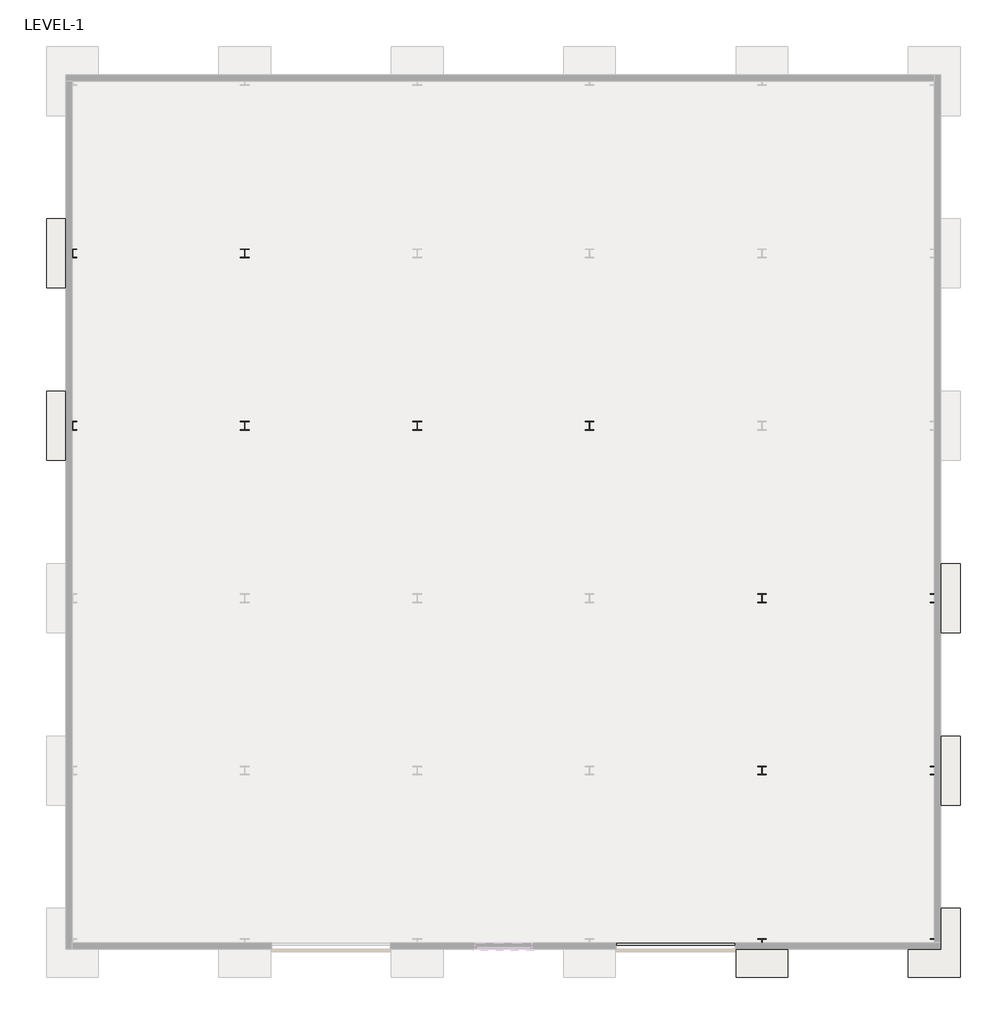
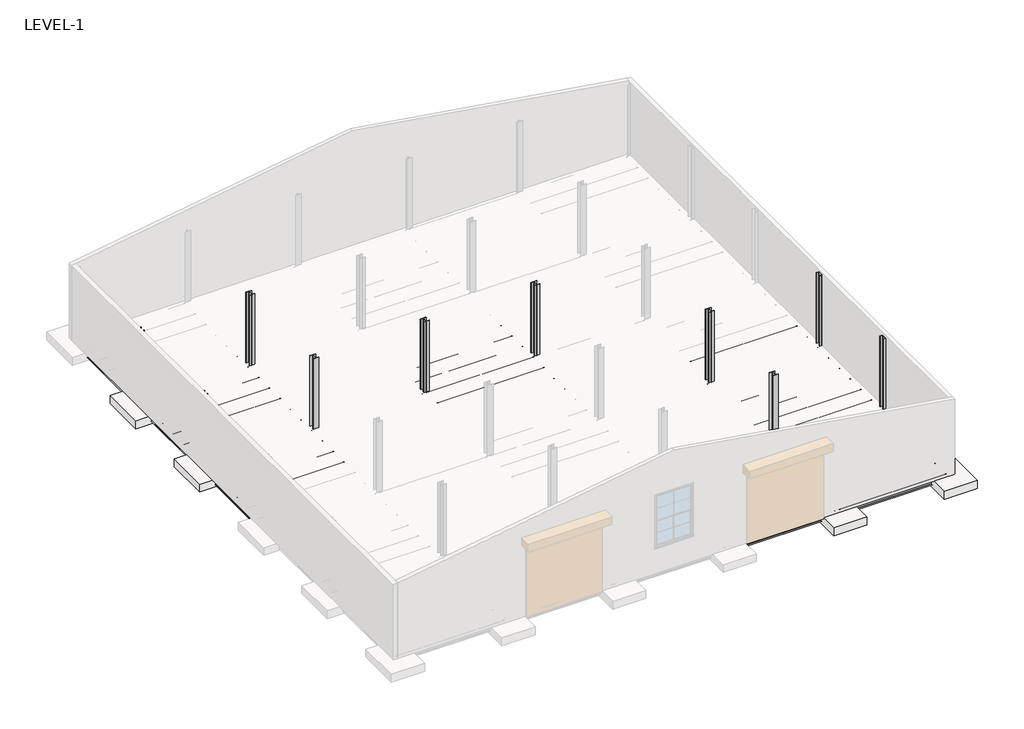
# One storey, part 2 of 3: 70 beams, 12 columns, 12 slabs.
"""IFC4 building model written with IfcOpenShell, lengths in millimetres."""

from ifc_helpers import new_model, si_unit, origin, place, context, project, spatial, transform, mapped, element, save
from components import ub_universal_beams_ub305x165x40_15f88fa9, ub_universal_beams_ub305x165x40_f918ae41, ub_universal_beams_ub305x165x40_f15b2736, ub_universal_beams_ub305x165x40_694d595e, ub_universal_beams_ub305x165x40_db4e7ae9, uc_universal_columns_column_uc305x305x97_11a20181, slab_7b69f09a

model = new_model("IFC4")

# Units and contexts
model_context = context("Model", 3, world=origin())
ifc_project = project(units=[si_unit("LENGTHUNIT", "METRE", prefix="MILLI")], contexts=[model_context])

# Site, building, storey
site = spatial("IfcSite", under=ifc_project)
building = spatial("IfcBuilding", under=site)
storey = spatial("IfcBuildingStorey", under=building, Name="LEVEL-1", Elevation=0.0)

# Beams
placement = place(None, origin())
ub_universal_beams_ub305x165x40_shape = ub_universal_beams_ub305x165x40_15f88fa9(model_context)
element("IfcBeam", 1, ObjectType="UB-Universal Beams : UB305x165x40", at=placement, inside=storey, context=model_context, shape_type="MappedRepresentation", body=[
    mapped(ub_universal_beams_ub305x165x40_shape, transform((-15492.3332854, 11071.5234105, -151.7), x_axis=(1.0, 0.0, 0.0), y_axis=(0.0, 1.0, 0.0), z_axis=(0.0, 0.0, 1.0))),
])
element("IfcBeam", 2, ObjectType="UB-Universal Beams : UB305x165x40", at=placement, inside=storey, context=model_context, shape_type="MappedRepresentation", body=[
    mapped(ub_universal_beams_ub305x165x40_shape, transform((-15492.3332854, 9039.5234105, -151.7), x_axis=(1.0, 0.0, 0.0), y_axis=(0.0, 1.0, 0.0), z_axis=(0.0, 0.0, 1.0))),
])
element("IfcBeam", 3, ObjectType="UB-Universal Beams : UB305x165x40", at=placement, inside=storey, context=model_context, shape_type="MappedRepresentation", body=[
    mapped(ub_universal_beams_ub305x165x40_shape, transform((-15492.3332854, 8023.5234105, -151.7), x_axis=(1.0, 0.0, 0.0), y_axis=(0.0, 1.0, 0.0), z_axis=(0.0, 0.0, 1.0))),
])
element("IfcBeam", 4, ObjectType="UB-Universal Beams : UB305x165x40", at=placement, inside=storey, context=model_context, shape_type="MappedRepresentation", body=[
    mapped(ub_universal_beams_ub305x165x40_shape, transform((-15492.3332854, 7007.5234105, -151.7), x_axis=(1.0, 0.0, 0.0), y_axis=(0.0, 1.0, 0.0), z_axis=(0.0, 0.0, 1.0))),
])
element("IfcBeam", 5, ObjectType="UB-Universal Beams : UB305x165x40", at=placement, inside=storey, context=model_context, shape_type="MappedRepresentation", body=[
    mapped(ub_universal_beams_ub305x165x40_shape, transform((-15492.3332854, 5991.5234105, -151.7), x_axis=(1.0, 0.0, 0.0), y_axis=(0.0, 1.0, 0.0), z_axis=(0.0, 0.0, 1.0))),
])
element("IfcBeam", 6, ObjectType="UB-Universal Beams : UB305x165x40", at=placement, inside=storey, context=model_context, shape_type="MappedRepresentation", body=[
    mapped(ub_universal_beams_ub305x165x40_shape, transform((-15492.3332854, 4975.5234105, -151.7), x_axis=(1.0, 0.0, 0.0), y_axis=(0.0, 1.0, 0.0), z_axis=(0.0, 0.0, 1.0))),
])
element("IfcBeam", 7, ObjectType="UB-Universal Beams : UB305x165x40", at=placement, inside=storey, context=model_context, shape_type="MappedRepresentation", body=[
    mapped(ub_universal_beams_ub305x165x40_shape, transform((-15492.3332854, 2943.5234105, -151.7), x_axis=(1.0, 0.0, 0.0), y_axis=(0.0, 1.0, 0.0), z_axis=(0.0, 0.0, 1.0))),
])
element("IfcBeam", 8, ObjectType="UB-Universal Beams : UB305x165x40", at=placement, inside=storey, context=model_context, shape_type="MappedRepresentation", body=[
    mapped(ub_universal_beams_ub305x165x40_shape, transform((-15492.3332854, 1927.5234105, -151.7), x_axis=(1.0, 0.0, 0.0), y_axis=(0.0, 1.0, 0.0), z_axis=(0.0, 0.0, 1.0))),
])
element("IfcBeam", 9, ObjectType="UB-Universal Beams : UB305x165x40", at=placement, inside=storey, context=model_context, shape_type="MappedRepresentation", body=[
    mapped(ub_universal_beams_ub305x165x40_shape, transform((-15492.3332854, 911.5234105, -151.7), x_axis=(1.0, 0.0, 0.0), y_axis=(0.0, 1.0, 0.0), z_axis=(0.0, 0.0, 1.0))),
])
element("IfcBeam", 10, ObjectType="UB-Universal Beams : UB305x165x40", at=placement, inside=storey, context=model_context, shape_type="MappedRepresentation", body=[
    mapped(ub_universal_beams_ub305x165x40_shape, transform((-3300.3332854, 7007.5234105, -151.7), x_axis=(1.0, 0.0, 0.0), y_axis=(0.0, 1.0, 0.0), z_axis=(0.0, 0.0, 1.0))),
])
element("IfcBeam", 11, ObjectType="UB-Universal Beams : UB305x165x40", at=placement, inside=storey, context=model_context, shape_type="MappedRepresentation", body=[
    mapped(ub_universal_beams_ub305x165x40_shape, transform((-3300.3332854, 5991.5234105, -151.7), x_axis=(1.0, 0.0, 0.0), y_axis=(0.0, 1.0, 0.0), z_axis=(0.0, 0.0, 1.0))),
])
element("IfcBeam", 12, ObjectType="UB-Universal Beams : UB305x165x40", at=placement, inside=storey, context=model_context, shape_type="MappedRepresentation", body=[
    mapped(ub_universal_beams_ub305x165x40_shape, transform((-3300.3332854, 4975.5234105, -151.7), x_axis=(1.0, 0.0, 0.0), y_axis=(0.0, 1.0, 0.0), z_axis=(0.0, 0.0, 1.0))),
])
element("IfcBeam", 13, ObjectType="UB-Universal Beams : UB305x165x40", at=placement, inside=storey, context=model_context, shape_type="MappedRepresentation", body=[
    mapped(ub_universal_beams_ub305x165x40_shape, transform((-3300.3332854, 2943.5234105, -151.7), x_axis=(1.0, 0.0, 0.0), y_axis=(0.0, 1.0, 0.0), z_axis=(0.0, 0.0, 1.0))),
])
element("IfcBeam", 14, ObjectType="UB-Universal Beams : UB305x165x40", at=placement, inside=storey, context=model_context, shape_type="MappedRepresentation", body=[
    mapped(ub_universal_beams_ub305x165x40_shape, transform((-3300.3332854, 1927.5234105, -151.7), x_axis=(1.0, 0.0, 0.0), y_axis=(0.0, 1.0, 0.0), z_axis=(0.0, 0.0, 1.0))),
])
element("IfcBeam", 15, ObjectType="UB-Universal Beams : UB305x165x40", at=placement, inside=storey, context=model_context, shape_type="MappedRepresentation", body=[
    mapped(ub_universal_beams_ub305x165x40_shape, transform((-3300.3332854, 911.5234105, -151.7), x_axis=(1.0, 0.0, 0.0), y_axis=(0.0, 1.0, 0.0), z_axis=(0.0, 0.0, 1.0))),
])
element("IfcBeam", 16, ObjectType="UB-Universal Beams : UB305x165x40", at=placement, inside=storey, context=model_context, shape_type="MappedRepresentation", body=[
    mapped(ub_universal_beams_ub305x165x40_shape, transform((8891.6667146, -104.4765895, -151.7), x_axis=(1.0, 0.0, 0.0), y_axis=(0.0, 1.0, 0.0), z_axis=(0.0, 0.0, 1.0))),
])
element("IfcBeam", 17, ObjectType="UB-Universal Beams : UB305x165x40", at=placement, inside=storey, context=model_context, shape_type="MappedRepresentation", body=[
    mapped(ub_universal_beams_ub305x165x40_shape, transform((8891.6667146, -1120.4765895, -151.7), x_axis=(1.0, 0.0, 0.0), y_axis=(0.0, 1.0, 0.0), z_axis=(0.0, 0.0, 1.0))),
])
element("IfcBeam", 18, ObjectType="UB-Universal Beams : UB305x165x40", at=placement, inside=storey, context=model_context, shape_type="MappedRepresentation", body=[
    mapped(ub_universal_beams_ub305x165x40_shape, transform((8891.6667146, -3152.4765895, -151.7), x_axis=(1.0, 0.0, 0.0), y_axis=(0.0, 1.0, 0.0), z_axis=(0.0, 0.0, 1.0))),
])
element("IfcBeam", 19, ObjectType="UB-Universal Beams : UB305x165x40", at=placement, inside=storey, context=model_context, shape_type="MappedRepresentation", body=[
    mapped(ub_universal_beams_ub305x165x40_shape, transform((8891.6667146, -4168.4765895, -151.7), x_axis=(1.0, 0.0, 0.0), y_axis=(0.0, 1.0, 0.0), z_axis=(0.0, 0.0, 1.0))),
])
element("IfcBeam", 20, ObjectType="UB-Universal Beams : UB305x165x40", at=placement, inside=storey, context=model_context, shape_type="MappedRepresentation", body=[
    mapped(ub_universal_beams_ub305x165x40_shape, transform((8891.6667146, -5184.4765895, -151.7), x_axis=(1.0, 0.0, 0.0), y_axis=(0.0, 1.0, 0.0), z_axis=(0.0, 0.0, 1.0))),
])
element("IfcBeam", 21, ObjectType="UB-Universal Beams : UB305x165x40", at=placement, inside=storey, context=model_context, shape_type="MappedRepresentation", body=[
    mapped(ub_universal_beams_ub305x165x40_shape, transform((8891.6667146, -6200.4765895, -151.7), x_axis=(1.0, 0.0, 0.0), y_axis=(0.0, 1.0, 0.0), z_axis=(0.0, 0.0, 1.0))),
])
element("IfcBeam", 22, ObjectType="UB-Universal Beams : UB305x165x40", at=placement, inside=storey, context=model_context, shape_type="MappedRepresentation", body=[
    mapped(ub_universal_beams_ub305x165x40_shape, transform((8891.6667146, -7216.4765895, -151.7), x_axis=(1.0, 0.0, 0.0), y_axis=(0.0, 1.0, 0.0), z_axis=(0.0, 0.0, 1.0))),
])
element("IfcBeam", 23, ObjectType="UB-Universal Beams : UB305x165x40", at=placement, inside=storey, context=model_context, shape_type="MappedRepresentation", body=[
    mapped(ub_universal_beams_ub305x165x40_shape, transform((8891.6667146, -9248.4765895, -151.7), x_axis=(1.0, 0.0, 0.0), y_axis=(0.0, 1.0, 0.0), z_axis=(0.0, 0.0, 1.0))),
])
element("IfcBeam", 24, ObjectType="UB-Universal Beams : UB305x165x40", at=placement, inside=storey, context=model_context, shape_type="MappedRepresentation", body=[
    mapped(ub_universal_beams_ub305x165x40_shape, transform((8891.6667146, -10264.4765895, -151.7), x_axis=(1.0, 0.0, 0.0), y_axis=(0.0, 1.0, 0.0), z_axis=(0.0, 0.0, 1.0))),
])
element("IfcBeam", 25, ObjectType="UB-Universal Beams : UB305x165x40", at=placement, inside=storey, context=model_context, shape_type="MappedRepresentation", body=[
    mapped(ub_universal_beams_ub305x165x40_shape, transform((8891.6667146, -11280.4765895, -151.7), x_axis=(1.0, 0.0, 0.0), y_axis=(0.0, 1.0, 0.0), z_axis=(0.0, 0.0, 1.0))),
])
element("IfcBeam", 26, ObjectType="UB-Universal Beams : UB305x165x40", at=placement, inside=storey, context=model_context, shape_type="MappedRepresentation", body=[
    mapped(ub_universal_beams_ub305x165x40_shape, transform((8891.6667146, -12296.4765895, -151.7), x_axis=(1.0, 0.0, 0.0), y_axis=(0.0, 1.0, 0.0), z_axis=(0.0, 0.0, 1.0))),
])
element("IfcBeam", 27, ObjectType="UB-Universal Beams : UB305x165x40", at=placement, inside=storey, context=model_context, shape_type="MappedRepresentation", body=[
    mapped(ub_universal_beams_ub305x165x40_shape, transform((8891.6667146, -13312.4765895, -151.7), x_axis=(1.0, 0.0, 0.0), y_axis=(0.0, 1.0, 0.0), z_axis=(0.0, 0.0, 1.0))),
])
element("IfcBeam", 28, ObjectType="UB-Universal Beams : UB305x165x40", at=placement, inside=storey, context=model_context, shape_type="MappedRepresentation", body=[
    mapped(ub_universal_beams_ub305x165x40_shape, transform((-7364.3332854, 7007.5234105, -151.7), x_axis=(0.0, -1.0, 0.0), y_axis=(1.0, 0.0, 0.0), z_axis=(0.0, 0.0, 1.0))),
])
element("IfcBeam", 29, ObjectType="UB-Universal Beams : UB305x165x40", at=placement, inside=storey, context=model_context, shape_type="MappedRepresentation", body=[
    mapped(ub_universal_beams_ub305x165x40_shape, transform((-8380.3332854, 7007.5234105, -151.7), x_axis=(0.0, -1.0, 0.0), y_axis=(1.0, 0.0, 0.0), z_axis=(0.0, 0.0, 1.0))),
])
element("IfcBeam", 30, ObjectType="UB-Universal Beams : UB305x165x40", at=placement, inside=storey, context=model_context, shape_type="MappedRepresentation", body=[
    mapped(ub_universal_beams_ub305x165x40_shape, transform((-9396.3332854, 7007.5234105, -151.7), x_axis=(0.0, -1.0, 0.0), y_axis=(1.0, 0.0, 0.0), z_axis=(0.0, 0.0, 1.0))),
])
element("IfcBeam", 31, ObjectType="UB-Universal Beams : UB305x165x40", at=placement, inside=storey, context=model_context, shape_type="MappedRepresentation", body=[
    mapped(ub_universal_beams_ub305x165x40_shape, transform((-10412.3332854, 7007.5234105, -151.7), x_axis=(0.0, -1.0, 0.0), y_axis=(1.0, 0.0, 0.0), z_axis=(0.0, 0.0, 1.0))),
])
element("IfcBeam", 32, ObjectType="UB-Universal Beams : UB305x165x40", at=placement, inside=storey, context=model_context, shape_type="MappedRepresentation", body=[
    mapped(ub_universal_beams_ub305x165x40_shape, transform((-11428.3332854, 7007.5234105, -151.7), x_axis=(0.0, -1.0, 0.0), y_axis=(1.0, 0.0, 0.0), z_axis=(0.0, 0.0, 1.0))),
])
element("IfcBeam", 33, ObjectType="UB-Universal Beams : UB305x165x40", at=placement, inside=storey, context=model_context, shape_type="MappedRepresentation", body=[
    mapped(ub_universal_beams_ub305x165x40_shape, transform((-7364.3332854, 911.5234105, -151.7), x_axis=(0.0, -1.0, 0.0), y_axis=(1.0, 0.0, 0.0), z_axis=(0.0, 0.0, 1.0))),
])
element("IfcBeam", 34, ObjectType="UB-Universal Beams : UB305x165x40", at=placement, inside=storey, context=model_context, shape_type="MappedRepresentation", body=[
    mapped(ub_universal_beams_ub305x165x40_shape, transform((-8380.3332854, 911.5234105, -151.7), x_axis=(0.0, -1.0, 0.0), y_axis=(1.0, 0.0, 0.0), z_axis=(0.0, 0.0, 1.0))),
])
element("IfcBeam", 35, ObjectType="UB-Universal Beams : UB305x165x40", at=placement, inside=storey, context=model_context, shape_type="MappedRepresentation", body=[
    mapped(ub_universal_beams_ub305x165x40_shape, transform((-9396.3332854, 911.5234105, -151.7), x_axis=(0.0, -1.0, 0.0), y_axis=(1.0, 0.0, 0.0), z_axis=(0.0, 0.0, 1.0))),
])
element("IfcBeam", 36, ObjectType="UB-Universal Beams : UB305x165x40", at=placement, inside=storey, context=model_context, shape_type="MappedRepresentation", body=[
    mapped(ub_universal_beams_ub305x165x40_shape, transform((-10412.3332854, 911.5234105, -151.7), x_axis=(0.0, -1.0, 0.0), y_axis=(1.0, 0.0, 0.0), z_axis=(0.0, 0.0, 1.0))),
])
element("IfcBeam", 37, ObjectType="UB-Universal Beams : UB305x165x40", at=placement, inside=storey, context=model_context, shape_type="MappedRepresentation", body=[
    mapped(ub_universal_beams_ub305x165x40_shape, transform((-11428.3332854, 911.5234105, -151.7), x_axis=(0.0, -1.0, 0.0), y_axis=(1.0, 0.0, 0.0), z_axis=(0.0, 0.0, 1.0))),
])
element("IfcBeam", 38, ObjectType="UB-Universal Beams : UB305x165x40", at=placement, inside=storey, context=model_context, shape_type="MappedRepresentation", body=[
    mapped(ub_universal_beams_ub305x165x40_shape, transform((4827.6667146, -5184.4765895, -151.7), x_axis=(0.0, -1.0, 0.0), y_axis=(1.0, 0.0, 0.0), z_axis=(0.0, 0.0, 1.0))),
])
element("IfcBeam", 39, ObjectType="UB-Universal Beams : UB305x165x40", at=placement, inside=storey, context=model_context, shape_type="MappedRepresentation", body=[
    mapped(ub_universal_beams_ub305x165x40_shape, transform((3811.6667146, -5184.4765895, -151.7), x_axis=(0.0, -1.0, 0.0), y_axis=(1.0, 0.0, 0.0), z_axis=(0.0, 0.0, 1.0))),
])
element("IfcBeam", 40, ObjectType="UB-Universal Beams : UB305x165x40", at=placement, inside=storey, context=model_context, shape_type="MappedRepresentation", body=[
    mapped(ub_universal_beams_ub305x165x40_shape, transform((2795.6667146, -5184.4765895, -151.7), x_axis=(0.0, -1.0, 0.0), y_axis=(1.0, 0.0, 0.0), z_axis=(0.0, 0.0, 1.0))),
])
element("IfcBeam", 41, ObjectType="UB-Universal Beams : UB305x165x40", at=placement, inside=storey, context=model_context, shape_type="MappedRepresentation", body=[
    mapped(ub_universal_beams_ub305x165x40_shape, transform((1779.6667146, -5184.4765895, -151.7), x_axis=(0.0, -1.0, 0.0), y_axis=(1.0, 0.0, 0.0), z_axis=(0.0, 0.0, 1.0))),
])
element("IfcBeam", 42, ObjectType="UB-Universal Beams : UB305x165x40", at=placement, inside=storey, context=model_context, shape_type="MappedRepresentation", body=[
    mapped(ub_universal_beams_ub305x165x40_shape, transform((763.6667146, -5184.4765895, -151.7), x_axis=(0.0, -1.0, 0.0), y_axis=(1.0, 0.0, 0.0), z_axis=(0.0, 0.0, 1.0))),
])
element("IfcBeam", 43, ObjectType="UB-Universal Beams : UB305x165x40", at=placement, inside=storey, context=model_context, shape_type="MappedRepresentation", body=[
    mapped(ub_universal_beams_ub305x165x40_shape, transform((4827.6667146, -11280.4765895, -151.7), x_axis=(0.0, -1.0, 0.0), y_axis=(1.0, 0.0, 0.0), z_axis=(0.0, 0.0, 1.0))),
])
element("IfcBeam", 44, ObjectType="UB-Universal Beams : UB305x165x40", at=placement, inside=storey, context=model_context, shape_type="MappedRepresentation", body=[
    mapped(ub_universal_beams_ub305x165x40_shape, transform((3811.6667146, -11280.4765895, -151.7), x_axis=(0.0, -1.0, 0.0), y_axis=(1.0, 0.0, 0.0), z_axis=(0.0, 0.0, 1.0))),
])
element("IfcBeam", 45, ObjectType="UB-Universal Beams : UB305x165x40", at=placement, inside=storey, context=model_context, shape_type="MappedRepresentation", body=[
    mapped(ub_universal_beams_ub305x165x40_shape, transform((2795.6667146, -11280.4765895, -151.7), x_axis=(0.0, -1.0, 0.0), y_axis=(1.0, 0.0, 0.0), z_axis=(0.0, 0.0, 1.0))),
])
element("IfcBeam", 46, ObjectType="UB-Universal Beams : UB305x165x40", at=placement, inside=storey, context=model_context, shape_type="MappedRepresentation", body=[
    mapped(ub_universal_beams_ub305x165x40_shape, transform((1779.6667146, -11280.4765895, -151.7), x_axis=(0.0, -1.0, 0.0), y_axis=(1.0, 0.0, 0.0), z_axis=(0.0, 0.0, 1.0))),
])
element("IfcBeam", 47, ObjectType="UB-Universal Beams : UB305x165x40", at=placement, inside=storey, context=model_context, shape_type="MappedRepresentation", body=[
    mapped(ub_universal_beams_ub305x165x40_shape, transform((763.6667146, -11280.4765895, -151.7), x_axis=(0.0, -1.0, 0.0), y_axis=(1.0, 0.0, 0.0), z_axis=(0.0, 0.0, 1.0))),
])
element("IfcBeam", 48, ObjectType="UB-Universal Beams : UB305x165x40", at=placement, inside=storey, context=model_context, shape_type="MappedRepresentation", body=[
    mapped(ub_universal_beams_ub305x165x40_shape, transform((2795.6667146, -14328.4765895, -151.7), x_axis=(1.0, 0.0, 0.0), y_axis=(0.0, 1.0, 0.0), z_axis=(0.0, 0.0, 1.0))),
])
element("IfcBeam", 49, ObjectType="UB-Universal Beams : UB305x165x40", at=placement, inside=storey, context=model_context, shape_type="MappedRepresentation", body=[
    mapped(ub_universal_beams_ub305x165x40_shape, transform((8891.6667146, -14328.4765895, -151.7), x_axis=(1.0, 0.0, 0.0), y_axis=(0.0, 1.0, 0.0), z_axis=(0.0, 0.0, 1.0))),
])
element("IfcBeam", 50, ObjectType="UB-Universal Beams : UB305x165x40", at=placement, inside=storey, context=model_context, shape_type="MappedRepresentation", body=[
    mapped(ub_universal_beams_ub305x165x40_shape, transform((2795.6667146, -8232.4765895, -151.7), x_axis=(1.0, 0.0, 0.0), y_axis=(0.0, 1.0, 0.0), z_axis=(0.0, 0.0, 1.0))),
])
element("IfcBeam", 51, ObjectType="UB-Universal Beams : UB305x165x40", at=placement, inside=storey, context=model_context, shape_type="MappedRepresentation", body=[
    mapped(ub_universal_beams_ub305x165x40_shape, transform((8891.6667146, -8232.4765895, -151.7), x_axis=(1.0, 0.0, 0.0), y_axis=(0.0, 1.0, 0.0), z_axis=(0.0, 0.0, 1.0))),
])
element("IfcBeam", 52, ObjectType="UB-Universal Beams : UB305x165x40", at=placement, inside=storey, context=model_context, shape_type="MappedRepresentation", body=[
    mapped(ub_universal_beams_ub305x165x40_shape, transform((2795.6667146, -2136.4765895, -151.7), x_axis=(1.0, 0.0, 0.0), y_axis=(0.0, 1.0, 0.0), z_axis=(0.0, 0.0, 1.0))),
])
element("IfcBeam", 53, ObjectType="UB-Universal Beams : UB305x165x40", at=placement, inside=storey, context=model_context, shape_type="MappedRepresentation", body=[
    mapped(ub_universal_beams_ub305x165x40_shape, transform((8891.6667146, -2136.4765895, -151.7), x_axis=(1.0, 0.0, 0.0), y_axis=(0.0, 1.0, 0.0), z_axis=(0.0, 0.0, 1.0))),
])
element("IfcBeam", 54, ObjectType="UB-Universal Beams : UB305x165x40", at=placement, inside=storey, context=model_context, shape_type="MappedRepresentation", body=[
    mapped(ub_universal_beams_ub305x165x40_shape, transform((-9396.3332854, 3959.5234105, -151.7), x_axis=(1.0, 0.0, 0.0), y_axis=(0.0, 1.0, 0.0), z_axis=(0.0, 0.0, 1.0))),
])
element("IfcBeam", 55, ObjectType="UB-Universal Beams : UB305x165x40", at=placement, inside=storey, context=model_context, shape_type="MappedRepresentation", body=[
    mapped(ub_universal_beams_ub305x165x40_shape, transform((-3300.3332854, 3959.5234105, -151.7), x_axis=(1.0, 0.0, 0.0), y_axis=(0.0, 1.0, 0.0), z_axis=(0.0, 0.0, 1.0))),
])
element("IfcBeam", 56, ObjectType="UB-Universal Beams : UB305x165x40", at=placement, inside=storey, context=model_context, shape_type="MappedRepresentation", body=[
    mapped(ub_universal_beams_ub305x165x40_shape, transform((-18540.3332854, 911.5234105, -151.7), x_axis=(0.0, 1.0, 0.0), y_axis=(-1.0, 0.0, 0.0), z_axis=(0.0, 0.0, 1.0))),
])
element("IfcBeam", 57, ObjectType="UB-Universal Beams : UB305x165x40", at=placement, inside=storey, context=model_context, shape_type="MappedRepresentation", body=[
    mapped(ub_universal_beams_ub305x165x40_shape, transform((-18540.3332854, 7007.5234105, -151.7), x_axis=(0.0, 1.0, 0.0), y_axis=(-1.0, 0.0, 0.0), z_axis=(0.0, 0.0, 1.0))),
])
ub_universal_beams_ub305x165x40_2_shape = ub_universal_beams_ub305x165x40_f918ae41(model_context)
element("IfcBeam", 58, ObjectType="UB-Universal Beams : UB305x165x40", at=placement, inside=storey, context=model_context, shape_type="MappedRepresentation", body=[
    mapped(ub_universal_beams_ub305x165x40_2_shape, transform((11939.6667146, -5184.4765895, -151.7), x_axis=(0.0, 1.0, 0.0), y_axis=(-1.0, 0.0, 0.0), z_axis=(0.0, 0.0, 1.0))),
])
element("IfcBeam", 59, ObjectType="UB-Universal Beams : UB305x165x40", at=placement, inside=storey, context=model_context, shape_type="MappedRepresentation", body=[
    mapped(ub_universal_beams_ub305x165x40_2_shape, transform((5843.6667146, -5184.4765895, -151.7), x_axis=(0.0, 1.0, 0.0), y_axis=(-1.0, 0.0, 0.0), z_axis=(0.0, 0.0, 1.0))),
])
element("IfcBeam", 60, ObjectType="UB-Universal Beams : UB305x165x40", at=placement, inside=storey, context=model_context, shape_type="MappedRepresentation", body=[
    mapped(ub_universal_beams_ub305x165x40_2_shape, transform((-252.3332854, 911.5234105, -151.7), x_axis=(0.0, 1.0, 0.0), y_axis=(-1.0, 0.0, 0.0), z_axis=(0.0, 0.0, 1.0))),
])
element("IfcBeam", 61, ObjectType="UB-Universal Beams : UB305x165x40", at=placement, inside=storey, context=model_context, shape_type="MappedRepresentation", body=[
    mapped(ub_universal_beams_ub305x165x40_2_shape, transform((-252.3332854, 7007.5234105, -151.7), x_axis=(0.0, 1.0, 0.0), y_axis=(-1.0, 0.0, 0.0), z_axis=(0.0, 0.0, 1.0))),
])
element("IfcBeam", 62, ObjectType="UB-Universal Beams : UB305x165x40", at=placement, inside=storey, context=model_context, shape_type="MappedRepresentation", body=[
    mapped(ub_universal_beams_ub305x165x40_2_shape, transform((-6348.3332854, 911.5234105, -151.7), x_axis=(0.0, 1.0, 0.0), y_axis=(-1.0, 0.0, 0.0), z_axis=(0.0, 0.0, 1.0))),
])
element("IfcBeam", 63, ObjectType="UB-Universal Beams : UB305x165x40", at=placement, inside=storey, context=model_context, shape_type="MappedRepresentation", body=[
    mapped(ub_universal_beams_ub305x165x40_2_shape, transform((-6348.3332854, 7007.5234105, -151.7), x_axis=(0.0, 1.0, 0.0), y_axis=(-1.0, 0.0, 0.0), z_axis=(0.0, 0.0, 1.0))),
])
element("IfcBeam", 64, ObjectType="UB-Universal Beams : UB305x165x40", at=placement, inside=storey, context=model_context, shape_type="MappedRepresentation", body=[
    mapped(ub_universal_beams_ub305x165x40_2_shape, transform((-12444.3332854, 911.5234105, -151.7), x_axis=(0.0, 1.0, 0.0), y_axis=(-1.0, 0.0, 0.0), z_axis=(0.0, 0.0, 1.0))),
])
element("IfcBeam", 65, ObjectType="UB-Universal Beams : UB305x165x40", at=placement, inside=storey, context=model_context, shape_type="MappedRepresentation", body=[
    mapped(ub_universal_beams_ub305x165x40_2_shape, transform((-12444.3332854, 7007.5234105, -151.7), x_axis=(0.0, 1.0, 0.0), y_axis=(-1.0, 0.0, 0.0), z_axis=(0.0, 0.0, 1.0))),
])
ub_universal_beams_ub305x165x40_3_shape = ub_universal_beams_ub305x165x40_f15b2736(model_context)
element("IfcBeam", 66, ObjectType="UB-Universal Beams : UB305x165x40", at=placement, inside=storey, context=model_context, shape_type="MappedRepresentation", body=[
    mapped(ub_universal_beams_ub305x165x40_3_shape, transform((-15549.3308854, 3959.5234105, -151.7), x_axis=(1.0, 0.0, 0.0), y_axis=(0.0, 1.0, 0.0), z_axis=(0.0, 0.0, 1.0))),
])
element("IfcBeam", 67, ObjectType="UB-Universal Beams : UB305x165x40", at=placement, inside=storey, context=model_context, shape_type="MappedRepresentation", body=[
    mapped(ub_universal_beams_ub305x165x40_3_shape, transform((-15549.3308854, 10055.5234105, -151.7), x_axis=(1.0, 0.0, 0.0), y_axis=(0.0, 1.0, 0.0), z_axis=(0.0, 0.0, 1.0))),
])
ub_universal_beams_ub305x165x40_4_shape = ub_universal_beams_ub305x165x40_694d595e(model_context)
element("IfcBeam", 68, ObjectType="UB-Universal Beams : UB305x165x40", at=placement, inside=storey, context=model_context, shape_type="MappedRepresentation", body=[
    mapped(ub_universal_beams_ub305x165x40_4_shape, transform((11939.6667146, -11337.6265895, -151.7), x_axis=(0.0, 1.0, 0.0), y_axis=(-1.0, 0.0, 0.0), z_axis=(0.0, 0.0, 1.0))),
])
element("IfcBeam", 69, ObjectType="UB-Universal Beams : UB305x165x40", at=placement, inside=storey, context=model_context, shape_type="MappedRepresentation", body=[
    mapped(ub_universal_beams_ub305x165x40_4_shape, transform((5843.6667146, -11337.6265895, -151.7), x_axis=(0.0, 1.0, 0.0), y_axis=(-1.0, 0.0, 0.0), z_axis=(0.0, 0.0, 1.0))),
])
ub_universal_beams_ub305x165x40_5_shape = ub_universal_beams_ub305x165x40_db4e7ae9(model_context)
element("IfcBeam", 70, ObjectType="UB-Universal Beams : UB305x165x40", at=placement, inside=storey, context=model_context, shape_type="MappedRepresentation", body=[
    mapped(ub_universal_beams_ub305x165x40_5_shape, transform((-18540.3332854, 13160.6734105, -151.7), x_axis=(0.0, 1.0, 0.0), y_axis=(-1.0, 0.0, 0.0), z_axis=(0.0, 0.0, 1.0))),
])

# Columns
uc_universal_columns_column_uc305x305x97_shape = uc_universal_columns_column_uc305x305x97_11a20181(model_context)
element("IfcColumn", 71, ObjectType="UC-Universal Columns-Column : UC305x305x97", at=placement, inside=storey, context=model_context, shape_type="MappedRepresentation", body=[
    mapped(uc_universal_columns_column_uc305x305x97_shape, transform((11939.6667146, -14328.4765895, 0.0), x_axis=(1.0, 0.0, 0.0), y_axis=(0.0, 1.0, 0.0), z_axis=(0.0, 0.0, 1.0))),
])
element("IfcColumn", 72, ObjectType="UC-Universal Columns-Column : UC305x305x97", at=placement, inside=storey, context=model_context, shape_type="MappedRepresentation", body=[
    mapped(uc_universal_columns_column_uc305x305x97_shape, transform((5843.6667146, -14328.4765895, 0.0), x_axis=(1.0, 0.0, 0.0), y_axis=(0.0, 1.0, 0.0), z_axis=(0.0, 0.0, 1.0))),
])
element("IfcColumn", 73, ObjectType="UC-Universal Columns-Column : UC305x305x97", at=placement, inside=storey, context=model_context, shape_type="MappedRepresentation", body=[
    mapped(uc_universal_columns_column_uc305x305x97_shape, transform((11939.6667146, -8232.4765895, 0.0), x_axis=(1.0, 0.0, 0.0), y_axis=(0.0, 1.0, 0.0), z_axis=(0.0, 0.0, 1.0))),
])
element("IfcColumn", 74, ObjectType="UC-Universal Columns-Column : UC305x305x97", at=placement, inside=storey, context=model_context, shape_type="MappedRepresentation", body=[
    mapped(uc_universal_columns_column_uc305x305x97_shape, transform((5843.6667146, -8232.4765895, 0.0), x_axis=(1.0, 0.0, 0.0), y_axis=(0.0, 1.0, 0.0), z_axis=(0.0, 0.0, 1.0))),
])
element("IfcColumn", 75, ObjectType="UC-Universal Columns-Column : UC305x305x97", at=placement, inside=storey, context=model_context, shape_type="MappedRepresentation", body=[
    mapped(uc_universal_columns_column_uc305x305x97_shape, transform((11939.6667146, -2136.4765895, 0.0), x_axis=(1.0, 0.0, 0.0), y_axis=(0.0, 1.0, 0.0), z_axis=(0.0, 0.0, 1.0))),
])
element("IfcColumn", 76, ObjectType="UC-Universal Columns-Column : UC305x305x97", at=placement, inside=storey, context=model_context, shape_type="MappedRepresentation", body=[
    mapped(uc_universal_columns_column_uc305x305x97_shape, transform((5843.6667146, -2136.4765895, 0.0), x_axis=(1.0, 0.0, 0.0), y_axis=(0.0, 1.0, 0.0), z_axis=(0.0, 0.0, 1.0))),
])
element("IfcColumn", 77, ObjectType="UC-Universal Columns-Column : UC305x305x97", at=placement, inside=storey, context=model_context, shape_type="MappedRepresentation", body=[
    mapped(uc_universal_columns_column_uc305x305x97_shape, transform((-252.3332854, 3959.5234105, 0.0), x_axis=(1.0, 0.0, 0.0), y_axis=(0.0, 1.0, 0.0), z_axis=(0.0, 0.0, 1.0))),
])
element("IfcColumn", 78, ObjectType="UC-Universal Columns-Column : UC305x305x97", at=placement, inside=storey, context=model_context, shape_type="MappedRepresentation", body=[
    mapped(uc_universal_columns_column_uc305x305x97_shape, transform((-6348.3332854, 3959.5234105, 0.0), x_axis=(1.0, 0.0, 0.0), y_axis=(0.0, 1.0, 0.0), z_axis=(0.0, 0.0, 1.0))),
])
element("IfcColumn", 79, ObjectType="UC-Universal Columns-Column : UC305x305x97", at=placement, inside=storey, context=model_context, shape_type="MappedRepresentation", body=[
    mapped(uc_universal_columns_column_uc305x305x97_shape, transform((-12444.3332854, 3959.5234105, 0.0), x_axis=(1.0, 0.0, 0.0), y_axis=(0.0, 1.0, 0.0), z_axis=(0.0, 0.0, 1.0))),
])
element("IfcColumn", 80, ObjectType="UC-Universal Columns-Column : UC305x305x97", at=placement, inside=storey, context=model_context, shape_type="MappedRepresentation", body=[
    mapped(uc_universal_columns_column_uc305x305x97_shape, transform((-18540.3332854, 3959.5234105, 0.0), x_axis=(1.0, 0.0, 0.0), y_axis=(0.0, 1.0, 0.0), z_axis=(0.0, 0.0, 1.0))),
])
element("IfcColumn", 81, ObjectType="UC-Universal Columns-Column : UC305x305x97", at=placement, inside=storey, context=model_context, shape_type="MappedRepresentation", body=[
    mapped(uc_universal_columns_column_uc305x305x97_shape, transform((-12444.3332854, 10055.5234105, 0.0), x_axis=(1.0, 0.0, 0.0), y_axis=(0.0, 1.0, 0.0), z_axis=(0.0, 0.0, 1.0))),
])
element("IfcColumn", 82, ObjectType="UC-Universal Columns-Column : UC305x305x97", at=placement, inside=storey, context=model_context, shape_type="MappedRepresentation", body=[
    mapped(uc_universal_columns_column_uc305x305x97_shape, transform((-18540.3332854, 10055.5234105, 0.0), x_axis=(1.0, 0.0, 0.0), y_axis=(0.0, 1.0, 0.0), z_axis=(0.0, 0.0, 1.0))),
])

# Slabs
slab_shape = slab_7b69f09a(model_context)
element("IfcSlab", 83, ObjectType="Footing-Rectangular : 96\" x 72\" x 18\"", at=placement, inside=storey, context=model_context, shape_type="MappedRepresentation", body=[
    mapped(slab_shape, transform((11939.6667146, -14328.4765895, 0.0), x_axis=(1.0, 0.0, 0.0), y_axis=(0.0, 1.0, 0.0), z_axis=(0.0, 0.0, 1.0))),
])
element("IfcSlab", 84, ObjectType="Footing-Rectangular : 96\" x 72\" x 18\"", at=placement, inside=storey, context=model_context, shape_type="MappedRepresentation", body=[
    mapped(slab_shape, transform((5843.6667146, -14328.4765895, 0.0), x_axis=(1.0, 0.0, 0.0), y_axis=(0.0, 1.0, 0.0), z_axis=(0.0, 0.0, 1.0))),
])
element("IfcSlab", 85, ObjectType="Footing-Rectangular : 96\" x 72\" x 18\"", at=placement, inside=storey, context=model_context, shape_type="MappedRepresentation", body=[
    mapped(slab_shape, transform((11939.6667146, -8232.4765895, 0.0), x_axis=(1.0, 0.0, 0.0), y_axis=(0.0, 1.0, 0.0), z_axis=(0.0, 0.0, 1.0))),
])
element("IfcSlab", 86, ObjectType="Footing-Rectangular : 96\" x 72\" x 18\"", at=placement, inside=storey, context=model_context, shape_type="MappedRepresentation", body=[
    mapped(slab_shape, transform((5843.6667146, -8232.4765895, 0.0), x_axis=(1.0, 0.0, 0.0), y_axis=(0.0, 1.0, 0.0), z_axis=(0.0, 0.0, 1.0))),
])
element("IfcSlab", 87, ObjectType="Footing-Rectangular : 96\" x 72\" x 18\"", at=placement, inside=storey, context=model_context, shape_type="MappedRepresentation", body=[
    mapped(slab_shape, transform((11939.6667146, -2136.4765895, 0.0), x_axis=(1.0, 0.0, 0.0), y_axis=(0.0, 1.0, 0.0), z_axis=(0.0, 0.0, 1.0))),
])
element("IfcSlab", 88, ObjectType="Footing-Rectangular : 96\" x 72\" x 18\"", at=placement, inside=storey, context=model_context, shape_type="MappedRepresentation", body=[
    mapped(slab_shape, transform((5843.6667146, -2136.4765895, 0.0), x_axis=(1.0, 0.0, 0.0), y_axis=(0.0, 1.0, 0.0), z_axis=(0.0, 0.0, 1.0))),
])
element("IfcSlab", 89, ObjectType="Footing-Rectangular : 96\" x 72\" x 18\"", at=placement, inside=storey, context=model_context, shape_type="MappedRepresentation", body=[
    mapped(slab_shape, transform((-252.3332854, 3959.5234105, 0.0), x_axis=(1.0, 0.0, 0.0), y_axis=(0.0, 1.0, 0.0), z_axis=(0.0, 0.0, 1.0))),
])
element("IfcSlab", 90, ObjectType="Footing-Rectangular : 96\" x 72\" x 18\"", at=placement, inside=storey, context=model_context, shape_type="MappedRepresentation", body=[
    mapped(slab_shape, transform((-6348.3332854, 3959.5234105, 0.0), x_axis=(1.0, 0.0, 0.0), y_axis=(0.0, 1.0, 0.0), z_axis=(0.0, 0.0, 1.0))),
])
element("IfcSlab", 91, ObjectType="Footing-Rectangular : 96\" x 72\" x 18\"", at=placement, inside=storey, context=model_context, shape_type="MappedRepresentation", body=[
    mapped(slab_shape, transform((-12444.3332854, 3959.5234105, 0.0), x_axis=(1.0, 0.0, 0.0), y_axis=(0.0, 1.0, 0.0), z_axis=(0.0, 0.0, 1.0))),
])
element("IfcSlab", 92, ObjectType="Footing-Rectangular : 96\" x 72\" x 18\"", at=placement, inside=storey, context=model_context, shape_type="MappedRepresentation", body=[
    mapped(slab_shape, transform((-18540.3332854, 3959.5234105, 0.0), x_axis=(1.0, 0.0, 0.0), y_axis=(0.0, 1.0, 0.0), z_axis=(0.0, 0.0, 1.0))),
])
element("IfcSlab", 93, ObjectType="Footing-Rectangular : 96\" x 72\" x 18\"", at=placement, inside=storey, context=model_context, shape_type="MappedRepresentation", body=[
    mapped(slab_shape, transform((-12444.3332854, 10055.5234105, 0.0), x_axis=(1.0, 0.0, 0.0), y_axis=(0.0, 1.0, 0.0), z_axis=(0.0, 0.0, 1.0))),
])
element("IfcSlab", 94, ObjectType="Footing-Rectangular : 96\" x 72\" x 18\"", at=placement, inside=storey, context=model_context, shape_type="MappedRepresentation", body=[
    mapped(slab_shape, transform((-18540.3332854, 10055.5234105, 0.0), x_axis=(1.0, 0.0, 0.0), y_axis=(0.0, 1.0, 0.0), z_axis=(0.0, 0.0, 1.0))),
])

save(model, "model.ifc")

# Revit data of these elements
# Type "UB-Universal Beams : UB305x165x40"
#   Section Name Key = "UB305X165X40"
#   Width = 16.5 cm
#   Web Thickness = 0.6 cm
#   Web Fillet = 0.89 cm
#   Warping Constant = 164000.0 cm⁶
#   Torsional Moment of Inertia = 14.70 cm⁴
#   Section Area = 51.3 cm²
#   Plastic Modulus weak axis = 142.0 cm³
#   Plastic Modulus strong axis = 623.0 cm³
#   Nominal Weight = 40.2999 kgf/m
#   Moment of Inertia weak axis = 764.00 cm⁴
#   Moment of Inertia strong axis = 8503.00 cm⁴
#   Height = 30.34 cm
#   Flange Thickness = 1.02 cm
#   Elastic Modulus weak axis = 92.6 cm³
#   Elastic Modulus strong axis = 560.0 cm³
#   Centroid Vertical = 15.17 cm
#   Centroid Horizontal = 8.25 cm
#   Bolt Spacing = 9.0 cm
#   Length [instance default] = 1500 mm
#   Structural Material [instance default] = Metal - Steel 43-275
#   Type Comments = ""
#   Assembly Code = ""
# Type "UC-Universal Columns-Column : UC305x305x97"
#   Section Name Key = "UC305x305x97"
#   Width = 30.53 cm
#   Web Thickness = 0.99 cm
#   Web Fillet = 1.52 cm
#   Warping Constant = 1560000.0 cm⁶
#   Torsional Moment of Inertia = 91.20 cm⁴
#   Section Area = 123.0 cm²
#   Plastic Modulus weak axis = 726.0 cm³
#   Plastic Modulus strong axis = 1592.0 cm³
#   Nominal Weight = 96.8996 kgf/m
#   Moment of Inertia weak axis = 7308.00 cm⁴
#   Moment of Inertia strong axis = 22249.00 cm⁴
#   Height = 30.79 cm
#   Flange Thickness = 1.54 cm
#   Elastic Modulus weak axis = 479.0 cm³
#   Elastic Modulus strong axis = 1445.0 cm³
#   Centroid Vertical = 15.395 cm
#   Centroid Horizontal = 15.265 cm
#   Bolt Spacing = 14.0 cm
#   Structural Material [instance default] = Metal - Steel 43-275
#   Type Comments = ""
#   Assembly Code = ""
# Type "Footing-Rectangular : 96\" x 72\" x 18\""
#   Assembly Code = "A1010100"
#   Width = 1828.8 mm
#   Length = 2438.4 mm
#   Foundation Thickness = 457.2 mm
#   Structural Material [instance default] = Concrete, Cast-in-Place gray
# Elements 1, 2, 3, 4, 5, 6, 7, 8, 9, 10, 11, 12, 13, 14, 15, 16, 17, 18, 19, 20, 21, 22, 23, 24, 25, 26, 27, 28, 29, 30, 31, 32, 33, 34, 35, 36, 37, 38, 39, 40, 41, 42, 43, 44, 45, 46, 47, 48, 49, 50, 51, 52, 53, 54, 55, 56, 57, 58, 59, 60, 61, 62, 63, 64, 65, 66, 67, 68, 69, 70 (IfcBeam, "UB-Universal Beams : UB305x165x40")
#   Structural Material = Metal - Steel 43-275
#   Phase Created = New Construction
#   Materials on its faces: "Metal - Steel 43-275"
# Elements 71, 72, 73, 74, 75, 76, 77, 78, 79, 80, 81, 82 (IfcColumn, "UC-Universal Columns-Column : UC305x305x97")
#   Structural Material = Metal - Steel 43-275
#   Phase Created = New Construction
#   Materials on its faces: "Metal - Steel 43-275"
# Elements 83, 84, 85, 86, 87, 88, 89, 90, 91, 92, 93, 94 (IfcSlab, "Footing-Rectangular : 96\" x 72\" x 18\"")
#   Structural Material = Concrete, Cast-in-Place gray
#   Phase Created = New Construction
#   Materials on its faces: "Concrete, Cast-in-Place gray"
# Materials
#   "Metal - Steel 43-275": class "Metal", colour RGB 247 247 247, transparency 0, Cost = 0
#   "Concrete, Cast-in-Place gray": class "Concrete", colour RGB 192 192 192, transparency 0, Description = "Cast-in-place concrete", Cost = 0
